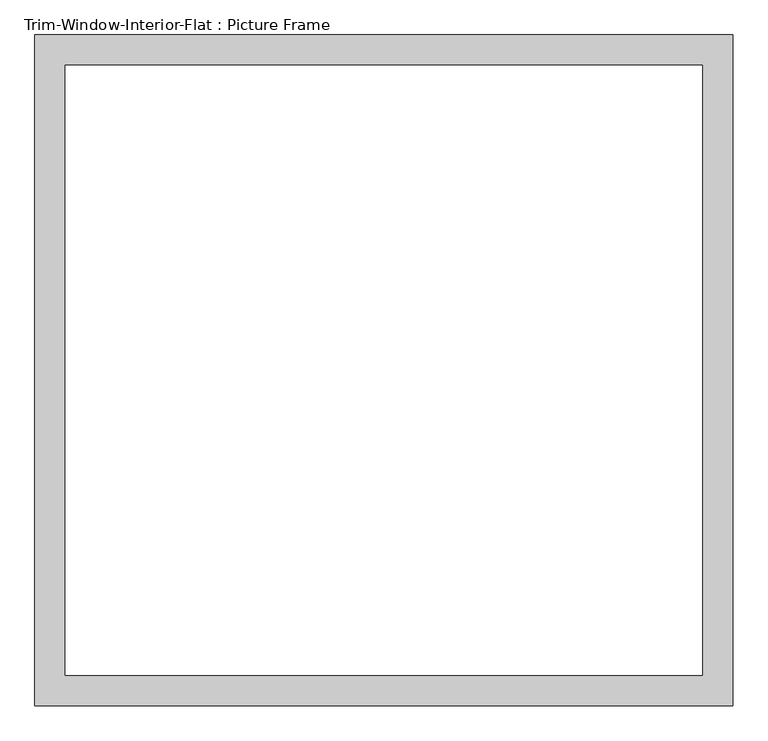
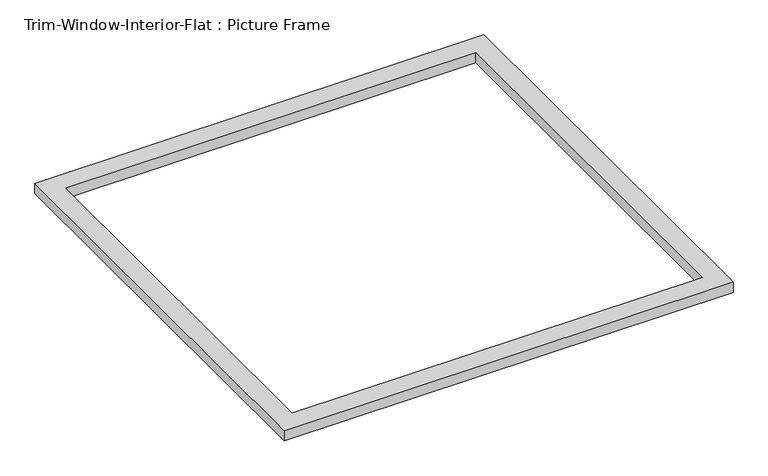
"""IFC4 building model written with IfcOpenShell, lengths in millimetres: proxy geometry, Trim-Window-Interior-Flat : Picture Frame."""

from ifc_helpers import new_model, si_unit, origin, origin_with_axes, place, context, project, spatial, polyline, outline, extrude, source, transform, mapped, element, save


def trim_window_interior_flat_picture_frame_8d0988b3(model_context):
    return source(origin(), model_context, "Body", "SweptSolid", [
        extrude(outline(polyline([(654.05, -44.45), (-654.05, -44.45), (-654.05, 1212.85), (654.05, 1212.85), (654.05, -44.45)]), holes=[polyline([(596.9, 12.7), (596.9, 1155.7), (-596.9, 1155.7), (-596.9, 12.7), (596.9, 12.7)])]), origin_with_axes(), (0.0, 0.0, 1.0), 31.75),
    ])


if __name__ == "__main__":
    model = new_model("IFC4")
    model_context = context("Model", 3, world=origin())
    ifc_project = project(units=[si_unit("LENGTHUNIT", "METRE", prefix="MILLI")], contexts=[model_context])
    site = spatial("IfcSite", under=ifc_project)
    building = spatial("IfcBuilding", under=site)
    placement = place(None, origin())
    trim_window_interior_flat_picture_frame_shape = trim_window_interior_flat_picture_frame_8d0988b3(model_context)
    element("IfcBuildingElementProxy", 1, Name="Trim-Window-Interior-Flat : Picture Frame", ObjectType="Trim-Window-Interior-Flat : Picture Frame", at=placement, inside=building, context=model_context, shape_type="MappedRepresentation", body=[
        mapped(trim_window_interior_flat_picture_frame_shape, transform((0.0, 0.0, 0.0), x_axis=(1.0, 0.0, 0.0), y_axis=(0.0, 1.0, 0.0), z_axis=(0.0, 0.0, 1.0))),
    ])
    save(model, "model.ifc")

# Revit data of these elements
# Type "Trim-Window-Interior-Flat : Picture Frame"
#   Trim Thickness_Picture Frame = 0' - 1 1/4"
#   Trim Width = 0' - 2 1/4"
#   Trim Thickness_with Sill = 0' - 0 3/4"
#   Sill Thickness = 0' - 1 1/4"
#   Opening Width [instance default] = 2' - 0"
#   Opening Height [instance default] = 3' - 0"
#   Default Elevation = 4' - 0"
#   Sill = no
#   Picture Frame = yes
#   Trim Material [instance default] = none
# Element 1 (IfcBuildingElementProxy, "Trim-Window-Interior-Flat : Picture Frame")
#   Opening Width = 4' - 0"
#   Opening Height = 3' - 10"
#   Trim Material = Wood - Stained
#   Materials on its faces: "Wood - Stained"
# Materials
#   "Wood - Stained": class "Wood", colour RGB 224 178 126, transparency 0, Cost = 0
